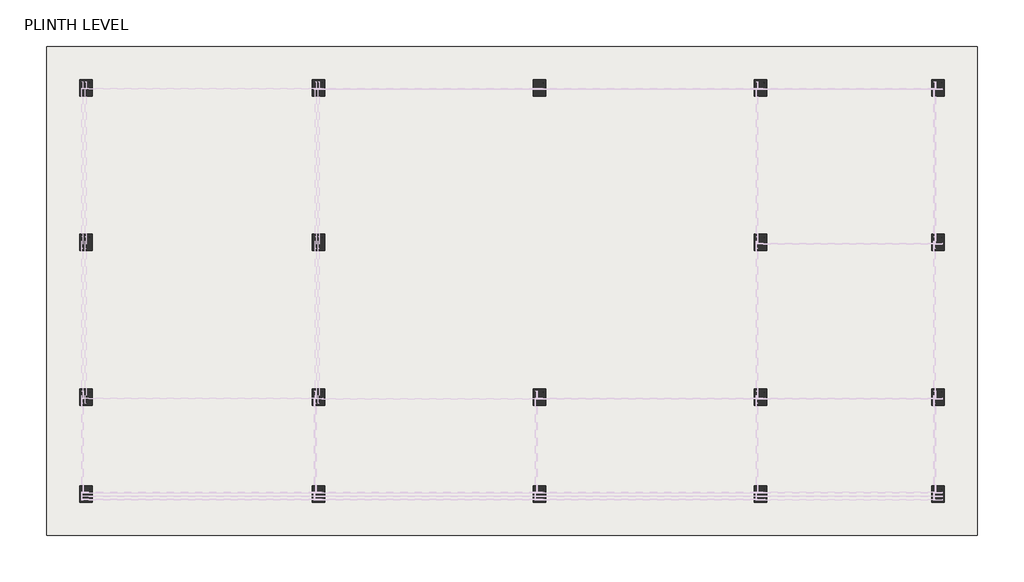
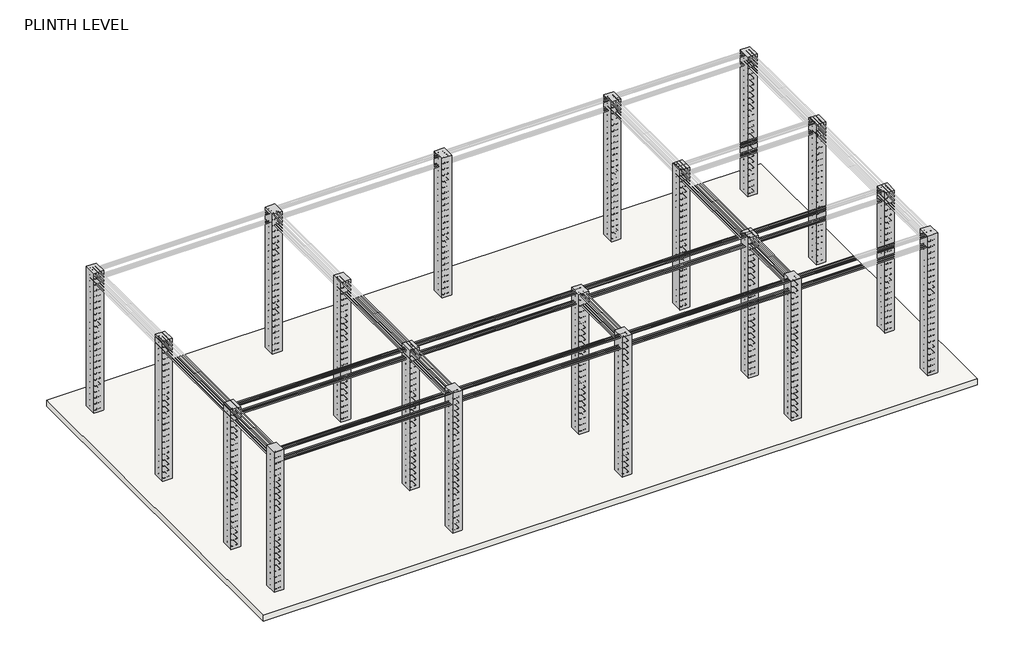
# One storey, part 1 of 6: 24 beams, 19 columns, 1 slab.
"""IFC4 building model written with IfcOpenShell, lengths in millimetres."""

from ifc_helpers import new_model, si_unit, frame, origin, origin_with_axes, place, context, project, spatial, polyline, outline, extrude, element, save

model = new_model("IFC4")

# Units and contexts
model_context = context("Model", 3, world=origin())
ifc_project = project(units=[si_unit("LENGTHUNIT", "METRE", prefix="MILLI")], contexts=[model_context])

# Site, building, storey
site = spatial("IfcSite", under=ifc_project)
building = spatial("IfcBuilding", under=site)
storey = spatial("IfcBuildingStorey", under=building, Name="PLINTH LEVEL", Elevation=0.0)

# Beams
placement = place(None, origin())
element("IfcBeam", 1, ObjectType="M_Concrete-Rectangular Beam : 230 x 300mm", at=placement, inside=storey, context=model_context, shape_type="SweptSolid", body=[
    extrude(outline(polyline([(-2504.7217857, -15209.6267376), (-2504.7217857, -14979.6267376), (1495.2782143, -14979.6267376), (1495.2782143, -15209.6267376), (-2504.7217857, -15209.6267376)])), frame((0.0, 0.0, -450.0), z_axis=(0.0, 0.0, 1.0), x_axis=(1.0, 0.0, 0.0)), (0.0, 0.0, 1.0), 300.0),
])
element("IfcBeam", 2, ObjectType="M_Concrete-Rectangular Beam : 230 x 300mm", at=placement, inside=storey, context=model_context, shape_type="SweptSolid", body=[
    extrude(outline(polyline([(1725.2782143, -15209.6267376), (1725.2782143, -14979.6267376), (5510.2782143, -14979.6267376), (5510.2782143, -15209.6267376), (1725.2782143, -15209.6267376)])), frame((0.0, 0.0, -450.0), z_axis=(0.0, 0.0, 1.0), x_axis=(1.0, 0.0, 0.0)), (0.0, 0.0, 1.0), 300.0),
])
element("IfcBeam", 3, ObjectType="M_Concrete-Rectangular Beam : 230 x 300mm", at=placement, inside=storey, context=model_context, shape_type="SweptSolid", body=[
    extrude(outline(polyline([(5740.2782143, -15209.6267376), (5740.2782143, -14979.6267376), (9525.2782143, -14979.6267376), (9525.2782143, -15209.6267376), (5740.2782143, -15209.6267376)])), frame((0.0, 0.0, -450.0), z_axis=(0.0, 0.0, 1.0), x_axis=(1.0, 0.0, 0.0)), (0.0, 0.0, 1.0), 300.0),
])
element("IfcBeam", 4, ObjectType="M_Concrete-Rectangular Beam : 230 x 300mm", at=placement, inside=storey, context=model_context, shape_type="SweptSolid", body=[
    extrude(outline(polyline([(9755.2782143, -15209.6267376), (9755.2782143, -14979.6267376), (12755.2782143, -14979.6267376), (12755.2782143, -15209.6267376), (9755.2782143, -15209.6267376)])), frame((0.0, 0.0, -450.0), z_axis=(0.0, 0.0, 1.0), x_axis=(1.0, 0.0, 0.0)), (0.0, 0.0, 1.0), 300.0),
])
element("IfcBeam", 5, ObjectType="M_Concrete-Rectangular Beam : 230 x 300mm", at=placement, inside=storey, context=model_context, shape_type="SweptSolid", body=[
    extrude(outline(polyline([(-2504.7217857, -13444.6267376), (-2504.7217857, -13214.6267376), (1495.2782143, -13214.6267376), (1495.2782143, -13444.6267376), (-2504.7217857, -13444.6267376)])), frame((0.0, 0.0, -450.0), z_axis=(0.0, 0.0, 1.0), x_axis=(1.0, 0.0, 0.0)), (0.0, 0.0, 1.0), 300.0),
])
element("IfcBeam", 6, ObjectType="M_Concrete-Rectangular Beam : 230 x 300mm", at=placement, inside=storey, context=model_context, shape_type="SweptSolid", body=[
    extrude(outline(polyline([(1725.2782143, -13444.6267376), (1725.2782143, -13214.6267376), (5510.2782143, -13214.6267376), (5510.2782143, -13444.6267376), (1725.2782143, -13444.6267376)])), frame((0.0, 0.0, -450.0), z_axis=(0.0, 0.0, 1.0), x_axis=(1.0, 0.0, 0.0)), (0.0, 0.0, 1.0), 300.0),
])
element("IfcBeam", 7, ObjectType="M_Concrete-Rectangular Beam : 230 x 300mm", at=placement, inside=storey, context=model_context, shape_type="SweptSolid", body=[
    extrude(outline(polyline([(5740.2782143, -13444.6267376), (5740.2782143, -13214.6267376), (9525.2782143, -13214.6267376), (9525.2782143, -13444.6267376), (5740.2782143, -13444.6267376)])), frame((0.0, 0.0, -450.0), z_axis=(0.0, 0.0, 1.0), x_axis=(1.0, 0.0, 0.0)), (0.0, 0.0, 1.0), 300.0),
])
element("IfcBeam", 8, ObjectType="M_Concrete-Rectangular Beam : 230 x 300mm", at=placement, inside=storey, context=model_context, shape_type="SweptSolid", body=[
    extrude(outline(polyline([(9755.2782143, -13444.6267376), (9755.2782143, -13214.6267376), (12755.2782143, -13214.6267376), (12755.2782143, -13444.6267376), (9755.2782143, -13444.6267376)])), frame((0.0, 0.0, -450.0), z_axis=(0.0, 0.0, 1.0), x_axis=(1.0, 0.0, 0.0)), (0.0, 0.0, 1.0), 300.0),
])
element("IfcBeam", 9, ObjectType="M_Concrete-Rectangular Beam : 230 x 300mm", at=placement, inside=storey, context=model_context, shape_type="SweptSolid", body=[
    extrude(outline(polyline([(-2504.7217857, -10629.6267376), (-2504.7217857, -10399.6267376), (1495.2782143, -10399.6267376), (1495.2782143, -10629.6267376), (-2504.7217857, -10629.6267376)])), frame((0.0, 0.0, -450.0), z_axis=(0.0, 0.0, 1.0), x_axis=(1.0, 0.0, 0.0)), (0.0, 0.0, 1.0), 300.0),
])
element("IfcBeam", 10, ObjectType="M_Concrete-Rectangular Beam : 230 x 300mm", at=placement, inside=storey, context=model_context, shape_type="SweptSolid", body=[
    extrude(outline(polyline([(9755.2782143, -10629.6267376), (9755.2782143, -10399.6267376), (12755.2782143, -10399.6267376), (12755.2782143, -10629.6267376), (9755.2782143, -10629.6267376)])), frame((0.0, 0.0, -450.0), z_axis=(0.0, 0.0, 1.0), x_axis=(1.0, 0.0, 0.0)), (0.0, 0.0, 1.0), 300.0),
])
element("IfcBeam", 11, ObjectType="M_Concrete-Rectangular Beam : 230 x 300mm", at=placement, inside=storey, context=model_context, shape_type="SweptSolid", body=[
    extrude(outline(polyline([(-2504.7217857, -7814.6267376), (-2504.7217857, -7584.6267376), (1495.2782143, -7584.6267376), (1495.2782143, -7814.6267376), (-2504.7217857, -7814.6267376)])), frame((0.0, 0.0, -450.0), z_axis=(0.0, 0.0, 1.0), x_axis=(1.0, 0.0, 0.0)), (0.0, 0.0, 1.0), 300.0),
])
element("IfcBeam", 12, ObjectType="M_Concrete-Rectangular Beam : 230 x 300mm", at=placement, inside=storey, context=model_context, shape_type="SweptSolid", body=[
    extrude(outline(polyline([(1725.2782143, -7814.6267376), (1725.2782143, -7584.6267376), (5510.2782143, -7584.6267376), (5510.2782143, -7814.6267376), (1725.2782143, -7814.6267376)])), frame((0.0, 0.0, -450.0), z_axis=(0.0, 0.0, 1.0), x_axis=(1.0, 0.0, 0.0)), (0.0, 0.0, 1.0), 300.0),
])
element("IfcBeam", 13, ObjectType="M_Concrete-Rectangular Beam : 230 x 300mm", at=placement, inside=storey, context=model_context, shape_type="SweptSolid", body=[
    extrude(outline(polyline([(5740.2782143, -7814.6267376), (5740.2782143, -7584.6267376), (9525.2782143, -7584.6267376), (9525.2782143, -7814.6267376), (5740.2782143, -7814.6267376)])), frame((0.0, 0.0, -450.0), z_axis=(0.0, 0.0, 1.0), x_axis=(1.0, 0.0, 0.0)), (0.0, 0.0, 1.0), 300.0),
])
element("IfcBeam", 14, ObjectType="M_Concrete-Rectangular Beam : 230 x 300mm", at=placement, inside=storey, context=model_context, shape_type="SweptSolid", body=[
    extrude(outline(polyline([(9755.2782143, -7814.6267376), (9755.2782143, -7584.6267376), (12755.2782143, -7584.6267376), (12755.2782143, -7814.6267376), (9755.2782143, -7814.6267376)])), frame((0.0, 0.0, -450.0), z_axis=(0.0, 0.0, 1.0), x_axis=(1.0, 0.0, 0.0)), (0.0, 0.0, 1.0), 300.0),
])
element("IfcBeam", 15, ObjectType="M_Concrete-Rectangular Beam : 230 x 300mm", at=placement, inside=storey, context=model_context, shape_type="SweptSolid", body=[
    extrude(outline(polyline([(-2504.7217857, -10364.6267376), (-2734.7217857, -10364.6267376), (-2734.7217857, -7849.6267376), (-2504.7217857, -7849.6267376), (-2504.7217857, -10364.6267376)])), frame((0.0, 0.0, -450.0), z_axis=(0.0, 0.0, 1.0), x_axis=(1.0, 0.0, 0.0)), (0.0, 0.0, 1.0), 300.0),
])
element("IfcBeam", 16, ObjectType="M_Concrete-Rectangular Beam : 230 x 300mm", at=placement, inside=storey, context=model_context, shape_type="SweptSolid", body=[
    extrude(outline(polyline([(-2504.7217857, -13179.6267376), (-2734.7217857, -13179.6267376), (-2734.7217857, -10664.6267376), (-2504.7217857, -10664.6267376), (-2504.7217857, -13179.6267376)])), frame((0.0, 0.0, -450.0), z_axis=(0.0, 0.0, 1.0), x_axis=(1.0, 0.0, 0.0)), (0.0, 0.0, 1.0), 300.0),
])
element("IfcBeam", 17, ObjectType="M_Concrete-Rectangular Beam : 230 x 300mm", at=placement, inside=storey, context=model_context, shape_type="SweptSolid", body=[
    extrude(outline(polyline([(-2504.7217857, -14944.6267376), (-2734.7217857, -14944.6267376), (-2734.7217857, -13479.6267376), (-2504.7217857, -13479.6267376), (-2504.7217857, -14944.6267376)])), frame((0.0, 0.0, -450.0), z_axis=(0.0, 0.0, 1.0), x_axis=(1.0, 0.0, 0.0)), (0.0, 0.0, 1.0), 300.0),
])
element("IfcBeam", 18, ObjectType="M_Concrete-Rectangular Beam : 230 x 300mm", at=placement, inside=storey, context=model_context, shape_type="SweptSolid", body=[
    extrude(outline(polyline([(1725.2782143, -10364.6267376), (1495.2782143, -10364.6267376), (1495.2782143, -7849.6267376), (1725.2782143, -7849.6267376), (1725.2782143, -10364.6267376)])), frame((0.0, 0.0, -450.0), z_axis=(0.0, 0.0, 1.0), x_axis=(1.0, 0.0, 0.0)), (0.0, 0.0, 1.0), 300.0),
])
element("IfcBeam", 19, ObjectType="M_Concrete-Rectangular Beam : 230 x 300mm", at=placement, inside=storey, context=model_context, shape_type="SweptSolid", body=[
    extrude(outline(polyline([(1725.2782143, -13179.6267376), (1495.2782143, -13179.6267376), (1495.2782143, -10664.6267376), (1725.2782143, -10664.6267376), (1725.2782143, -13179.6267376)])), frame((0.0, 0.0, -450.0), z_axis=(0.0, 0.0, 1.0), x_axis=(1.0, 0.0, 0.0)), (0.0, 0.0, 1.0), 300.0),
])
element("IfcBeam", 20, ObjectType="M_Concrete-Rectangular Beam : 230 x 300mm", at=placement, inside=storey, context=model_context, shape_type="SweptSolid", body=[
    extrude(outline(polyline([(9755.2782143, -10364.6267376), (9525.2782143, -10364.6267376), (9525.2782143, -7849.6267376), (9755.2782143, -7849.6267376), (9755.2782143, -10364.6267376)])), frame((0.0, 0.0, -450.0), z_axis=(0.0, 0.0, 1.0), x_axis=(1.0, 0.0, 0.0)), (0.0, 0.0, 1.0), 300.0),
])
element("IfcBeam", 21, ObjectType="M_Concrete-Rectangular Beam : 230 x 300mm", at=placement, inside=storey, context=model_context, shape_type="SweptSolid", body=[
    extrude(outline(polyline([(9755.2782143, -13179.6267376), (9525.2782143, -13179.6267376), (9525.2782143, -10664.6267376), (9755.2782143, -10664.6267376), (9755.2782143, -13179.6267376)])), frame((0.0, 0.0, -450.0), z_axis=(0.0, 0.0, 1.0), x_axis=(1.0, 0.0, 0.0)), (0.0, 0.0, 1.0), 300.0),
])
element("IfcBeam", 22, ObjectType="M_Concrete-Rectangular Beam : 230 x 300mm", at=placement, inside=storey, context=model_context, shape_type="SweptSolid", body=[
    extrude(outline(polyline([(12985.2782143, -10364.6267376), (12755.2782143, -10364.6267376), (12755.2782143, -7849.6267376), (12985.2782143, -7849.6267376), (12985.2782143, -10364.6267376)])), frame((0.0, 0.0, -450.0), z_axis=(0.0, 0.0, 1.0), x_axis=(1.0, 0.0, 0.0)), (0.0, 0.0, 1.0), 300.0),
])
element("IfcBeam", 23, ObjectType="M_Concrete-Rectangular Beam : 230 x 300mm", at=placement, inside=storey, context=model_context, shape_type="SweptSolid", body=[
    extrude(outline(polyline([(12985.2782143, -13179.6267376), (12755.2782143, -13179.6267376), (12755.2782143, -10664.6267376), (12985.2782143, -10664.6267376), (12985.2782143, -13179.6267376)])), frame((0.0, 0.0, -450.0), z_axis=(0.0, 0.0, 1.0), x_axis=(1.0, 0.0, 0.0)), (0.0, 0.0, 1.0), 300.0),
])
element("IfcBeam", 24, ObjectType="M_Concrete-Rectangular Beam : 230 x 300mm", at=placement, inside=storey, context=model_context, shape_type="SweptSolid", body=[
    extrude(outline(polyline([(12985.2782143, -14944.6267376), (12755.2782143, -14944.6267376), (12755.2782143, -13479.6267376), (12985.2782143, -13479.6267376), (12985.2782143, -14944.6267376)])), frame((0.0, 0.0, -450.0), z_axis=(0.0, 0.0, 1.0), x_axis=(1.0, 0.0, 0.0)), (0.0, 0.0, 1.0), 300.0),
])

# Columns
element("IfcColumn", 25, ObjectType="M_Concrete-Rectangular-Column : 230 x 300mm 2", at=placement, inside=storey, context=model_context, shape_type="SweptSolid", body=[
    extrude(outline(polyline([(-2504.7217857, -14944.6267376), (-2504.7217857, -15244.6267376), (-2734.7217857, -15244.6267376), (-2734.7217857, -14944.6267376), (-2504.7217857, -14944.6267376)])), origin_with_axes(), (0.0, 0.0, 1.0), 3505.2),
])
element("IfcColumn", 26, ObjectType="M_Concrete-Rectangular-Column : 230 x 300mm 2", at=placement, inside=storey, context=model_context, shape_type="SweptSolid", body=[
    extrude(outline(polyline([(1725.2782143, -14944.6267376), (1725.2782143, -15244.6267376), (1495.2782143, -15244.6267376), (1495.2782143, -14944.6267376), (1725.2782143, -14944.6267376)])), origin_with_axes(), (0.0, 0.0, 1.0), 3505.2),
])
element("IfcColumn", 27, ObjectType="M_Concrete-Rectangular-Column : 230 x 300mm 2", at=placement, inside=storey, context=model_context, shape_type="SweptSolid", body=[
    extrude(outline(polyline([(5740.2782143, -14944.6267376), (5740.2782143, -15244.6267376), (5510.2782143, -15244.6267376), (5510.2782143, -14944.6267376), (5740.2782143, -14944.6267376)])), origin_with_axes(), (0.0, 0.0, 1.0), 3505.2),
])
element("IfcColumn", 28, ObjectType="M_Concrete-Rectangular-Column : 230 x 300mm 2", at=placement, inside=storey, context=model_context, shape_type="SweptSolid", body=[
    extrude(outline(polyline([(9755.2782143, -14944.6267376), (9755.2782143, -15244.6267376), (9525.2782143, -15244.6267376), (9525.2782143, -14944.6267376), (9755.2782143, -14944.6267376)])), origin_with_axes(), (0.0, 0.0, 1.0), 3505.2),
])
element("IfcColumn", 29, ObjectType="M_Concrete-Rectangular-Column : 230 x 300mm 2", at=placement, inside=storey, context=model_context, shape_type="SweptSolid", body=[
    extrude(outline(polyline([(12985.2782143, -14944.6267376), (12985.2782143, -15244.6267376), (12755.2782143, -15244.6267376), (12755.2782143, -14944.6267376), (12985.2782143, -14944.6267376)])), origin_with_axes(), (0.0, 0.0, 1.0), 3505.2),
])
element("IfcColumn", 30, ObjectType="M_Concrete-Rectangular-Column : 230 x 300mm 2", at=placement, inside=storey, context=model_context, shape_type="SweptSolid", body=[
    extrude(outline(polyline([(-2504.7217857, -13179.6267376), (-2504.7217857, -13479.6267376), (-2734.7217857, -13479.6267376), (-2734.7217857, -13179.6267376), (-2504.7217857, -13179.6267376)])), origin_with_axes(), (0.0, 0.0, 1.0), 3505.2),
])
element("IfcColumn", 31, ObjectType="M_Concrete-Rectangular-Column : 230 x 300mm 2", at=placement, inside=storey, context=model_context, shape_type="SweptSolid", body=[
    extrude(outline(polyline([(1725.2782143, -13179.6267376), (1725.2782143, -13479.6267376), (1495.2782143, -13479.6267376), (1495.2782143, -13179.6267376), (1725.2782143, -13179.6267376)])), origin_with_axes(), (0.0, 0.0, 1.0), 3505.2),
])
element("IfcColumn", 32, ObjectType="M_Concrete-Rectangular-Column : 230 x 300mm 2", at=placement, inside=storey, context=model_context, shape_type="SweptSolid", body=[
    extrude(outline(polyline([(5740.2782143, -13179.6267376), (5740.2782143, -13479.6267376), (5510.2782143, -13479.6267376), (5510.2782143, -13179.6267376), (5740.2782143, -13179.6267376)])), origin_with_axes(), (0.0, 0.0, 1.0), 3505.2),
])
element("IfcColumn", 33, ObjectType="M_Concrete-Rectangular-Column : 230 x 300mm 2", at=placement, inside=storey, context=model_context, shape_type="SweptSolid", body=[
    extrude(outline(polyline([(9755.2782143, -13179.6267376), (9755.2782143, -13479.6267376), (9525.2782143, -13479.6267376), (9525.2782143, -13179.6267376), (9755.2782143, -13179.6267376)])), origin_with_axes(), (0.0, 0.0, 1.0), 3505.2),
])
element("IfcColumn", 34, ObjectType="M_Concrete-Rectangular-Column : 230 x 300mm 2", at=placement, inside=storey, context=model_context, shape_type="SweptSolid", body=[
    extrude(outline(polyline([(12985.2782143, -13179.6267376), (12985.2782143, -13479.6267376), (12755.2782143, -13479.6267376), (12755.2782143, -13179.6267376), (12985.2782143, -13179.6267376)])), origin_with_axes(), (0.0, 0.0, 1.0), 3505.2),
])
element("IfcColumn", 35, ObjectType="M_Concrete-Rectangular-Column : 230 x 300mm 2", at=placement, inside=storey, context=model_context, shape_type="SweptSolid", body=[
    extrude(outline(polyline([(-2504.7217857, -10364.6267376), (-2504.7217857, -10664.6267376), (-2734.7217857, -10664.6267376), (-2734.7217857, -10364.6267376), (-2504.7217857, -10364.6267376)])), origin_with_axes(), (0.0, 0.0, 1.0), 3505.2),
])
element("IfcColumn", 36, ObjectType="M_Concrete-Rectangular-Column : 230 x 300mm 2", at=placement, inside=storey, context=model_context, shape_type="SweptSolid", body=[
    extrude(outline(polyline([(1725.2782143, -10364.6267376), (1725.2782143, -10664.6267376), (1495.2782143, -10664.6267376), (1495.2782143, -10364.6267376), (1725.2782143, -10364.6267376)])), origin_with_axes(), (0.0, 0.0, 1.0), 3505.2),
])
element("IfcColumn", 37, ObjectType="M_Concrete-Rectangular-Column : 230 x 300mm 2", at=placement, inside=storey, context=model_context, shape_type="SweptSolid", body=[
    extrude(outline(polyline([(9755.2782143, -10364.6267376), (9755.2782143, -10664.6267376), (9525.2782143, -10664.6267376), (9525.2782143, -10364.6267376), (9755.2782143, -10364.6267376)])), origin_with_axes(), (0.0, 0.0, 1.0), 3505.2),
])
element("IfcColumn", 38, ObjectType="M_Concrete-Rectangular-Column : 230 x 300mm 2", at=placement, inside=storey, context=model_context, shape_type="SweptSolid", body=[
    extrude(outline(polyline([(12985.2782143, -10364.6267376), (12985.2782143, -10664.6267376), (12755.2782143, -10664.6267376), (12755.2782143, -10364.6267376), (12985.2782143, -10364.6267376)])), origin_with_axes(), (0.0, 0.0, 1.0), 3505.2),
])
element("IfcColumn", 39, ObjectType="M_Concrete-Rectangular-Column : 230 x 300mm 2", at=placement, inside=storey, context=model_context, shape_type="SweptSolid", body=[
    extrude(outline(polyline([(-2504.7217857, -7549.6267376), (-2504.7217857, -7849.6267376), (-2734.7217857, -7849.6267376), (-2734.7217857, -7549.6267376), (-2504.7217857, -7549.6267376)])), origin_with_axes(), (0.0, 0.0, 1.0), 3505.2),
])
element("IfcColumn", 40, ObjectType="M_Concrete-Rectangular-Column : 230 x 300mm 2", at=placement, inside=storey, context=model_context, shape_type="SweptSolid", body=[
    extrude(outline(polyline([(1725.2782143, -7549.6267376), (1725.2782143, -7849.6267376), (1495.2782143, -7849.6267376), (1495.2782143, -7549.6267376), (1725.2782143, -7549.6267376)])), origin_with_axes(), (0.0, 0.0, 1.0), 3505.2),
])
element("IfcColumn", 41, ObjectType="M_Concrete-Rectangular-Column : 230 x 300mm 2", at=placement, inside=storey, context=model_context, shape_type="SweptSolid", body=[
    extrude(outline(polyline([(5740.2782143, -7549.6267376), (5740.2782143, -7849.6267376), (5510.2782143, -7849.6267376), (5510.2782143, -7549.6267376), (5740.2782143, -7549.6267376)])), origin_with_axes(), (0.0, 0.0, 1.0), 3505.2),
])
element("IfcColumn", 42, ObjectType="M_Concrete-Rectangular-Column : 230 x 300mm 2", at=placement, inside=storey, context=model_context, shape_type="SweptSolid", body=[
    extrude(outline(polyline([(9755.2782143, -7549.6267376), (9755.2782143, -7849.6267376), (9525.2782143, -7849.6267376), (9525.2782143, -7549.6267376), (9755.2782143, -7549.6267376)])), origin_with_axes(), (0.0, 0.0, 1.0), 3505.2),
])
element("IfcColumn", 43, ObjectType="M_Concrete-Rectangular-Column : 230 x 300mm 2", at=placement, inside=storey, context=model_context, shape_type="SweptSolid", body=[
    extrude(outline(polyline([(12985.2782143, -7549.6267376), (12985.2782143, -7849.6267376), (12755.2782143, -7849.6267376), (12755.2782143, -7549.6267376), (12985.2782143, -7549.6267376)])), origin_with_axes(), (0.0, 0.0, 1.0), 3505.2),
])

# Slab
element("IfcSlab", 44, ObjectType="Generic 150mm 2", at=placement, inside=storey, context=model_context, shape_type="SweptSolid", body=[
    extrude(outline(polyline([(13585.2782143, -6949.6267376), (13585.2782143, -15844.6267376), (-3334.7217857, -15844.6267376), (-3334.7217857, -6949.6267376), (13585.2782143, -6949.6267376)])), frame((0.0, 0.0, -150.0), z_axis=(0.0, 0.0, 1.0), x_axis=(1.0, 0.0, 0.0)), (0.0, 0.0, 1.0), 150.0),
])

save(model, "model.ifc")

# Revit data of these elements
# Type "M_Concrete-Rectangular Beam : 230 x 300mm"
#   Length [instance default] = 5' - 0"
#   b = 0' - 9.05512"
#   h = 0' - 11.81102"
#   Structural Material [instance default] = Concrete, Cast-in-Place gray
#   Assembly Code = ""
# Type "M_Concrete-Rectangular-Column : 230 x 300mm 2"
#   b = 0' - 9.05512"
#   h = 0' - 11.81102"
#   Structural Material [instance default] = Concrete, Cast-in-Place gray
# Type "Generic 150mm 2"
#   Function = 0
#   Layers, outside or top first: 0' - 5.90551" no material (function 1)
# Elements 1, 2, 3, 4, 5, 6, 7, 8, 9, 10, 11, 12, 13, 14, 15, 16, 17, 18, 19, 20, 21, 22, 23, 24 (IfcBeam, "M_Concrete-Rectangular Beam : 230 x 300mm")
#   Structural Material = Concrete, Cast-in-Place gray
#   Phase Created = New Construction
#   Materials on its faces: "Concrete, Cast-in-Place gray"
# Elements 25, 26, 27, 28, 29, 30, 31, 32, 33, 34, 35, 36, 37, 38, 39, 40, 41, 42, 43 (IfcColumn, "M_Concrete-Rectangular-Column : 230 x 300mm 2")
#   Structural Material = Concrete, Cast-in-Place gray
#   Phase Created = New Construction
#   Materials on its faces: "Concrete, Cast-in-Place gray"
# Element 44 (IfcSlab, "Generic 150mm 2")
#   Height Offset From Level = 0' - 0"
#   built-in parameter 1001954 = 1
#   Phase Created = New Construction
#   Materials on its faces: "Default Floor"
# Materials
#   "Concrete, Cast-in-Place gray": class "Concrete", colour RGB 192 192 192, transparency 0, Description = "Cast-in-place concrete", Cost = 0
#   "Default Floor": colour RGB 127 127 127, transparency 0, Cost = 0
